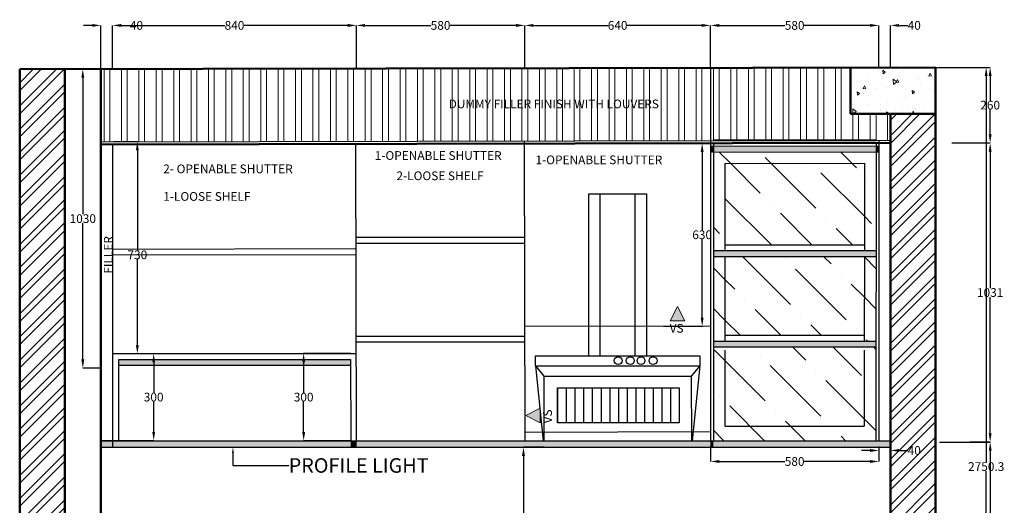
# Model space of a CAD drawing. Units: millimetres. Extents: x 26138 to 44889, y 15820 to 21179.
# Tile 4 of 8: x 31250 to 34642, y 17594 to 19266. Entities that reach past the tile are written whole.
import ezdxf
from ezdxf import colors
from ezdxf.entities.mleader import LeaderData, LeaderLine
from ezdxf.math import Vec2, Vec3

# ---------------------------------------------------------------- set-up
doc = ezdxf.new("R2010")
doc.units = ezdxf.units.MM
doc.header["$MEASUREMENT"] = 0
doc.header["$PDMODE"] = 3
for name, color, linetype, lineweight in [('A-ANNO-DIMS', 70, 'Continuous', 18), ('A-ANNO-SYMB', 1, 'Continuous', 18), ('A-ANNO-TEXT', 7, 'Continuous', 18), ('A-ELEV', 7, 'Continuous', 25), ('A-FURN-PATT', 40, 'Continuous', 13), ('A-WALL', 1, 'Continuous', 50), ('A-WALL-PATT', 8, 'Continuous', 13)]:
    doc.layers.add(name, color=color, linetype=linetype, lineweight=lineweight)
doc.styles.get("Standard").update_dxf_attribs({"font": 'arial.ttf'})
doc.dimstyles.get("Standard").update_dxf_attribs({"dimtxt": 30, "dimasz": 30, "dimexe": 0.18, "dimexo": 0.0625, "dimgap": 0.09, "dimtad": 0, "dimtih": 1, "dimtoh": 1, "dimdec": 0, "dimzin": 0, "dimdsep": 46, "dimtxsty": 'Standard', "dimcen": 0.09, "dimadec": 0, "dimazin": 0, "dimtfac": 1, "dimtdec": 0, "dimtofl": 0, "dimtmove": 0, "dimatfit": 3, "dimfxl": 1, "dimtolj": 1, "dimtzin": 0, "dimarcsym": 0})
pattern_1 = [(45, (-3504.08, -2261.207), (-39.77476, 39.77476), []), (45, (-3477.56, -2261.207), (-39.77476, 39.77476), [])]
pattern_2 = [(135, (-3504.08, -2261.21), (-192.02369, 52.3701), [246.875, -49.375, 0, -49.375])]
pattern_3 = [(90, (-379.65, -2261.21), (-60, 0), []), (90, (-359.65, -2241.21), (-60, 0), [])]

# ---------------------------------------------------------------- blocks, each defined once
blk = doc.blocks.new('*D40')
at = {"layer": 'A-ANNO-DIMS', "color": 0, "lineweight": -2, "transparency": 16777216}
for p, q in [((31499.9, 19246.8), (31469.9, 19246.8)), ((31529.9, 19096.4), (31529.9, 19247)), ((31569.9, 19096.4), (31569.9, 19247)), ((31599.9, 19246.8), (31629.9, 19246.8))]:
    blk.add_line(p, q, dxfattribs=at)
at = {"layer": 'A-ANNO-DIMS', "color": 0, "transparency": 16777216}
for points in [[(31499.9, 19251.8), (31499.9, 19241.8), (31529.9, 19246.8)], [(31599.9, 19251.8), (31599.9, 19241.8), (31569.9, 19246.8)]]:
    blk.add_solid(points, dxfattribs=at)
at = {"layer": 'Defpoints', "color": 0, "transparency": 16777216}
for p in [(31569.9, 19246.8), (31529.9, 19096.3), (31569.9, 19096.3)]:
    blk.add_point(p, dxfattribs=at)
at = {"layer": 'A-ANNO-DIMS', "color": 0, "transparency": 16777216, "insert": (31652, 19246.8), "char_height": 30, "attachment_point": 5}
blk.add_mtext('\\A1;40', dxfattribs=at)
blk = doc.blocks.new('*D41')
at = {"layer": 'A-ANNO-DIMS', "color": 0, "lineweight": -2, "transparency": 16777216}
for p, q in [((31569.9, 19096.5), (31569.9, 19247)), ((31599.9, 19246.8), (31956.7, 19246.8)), ((32379.9, 19246.8), (32023.1, 19246.8)), ((32409.9, 19096.5), (32409.9, 19247))]:
    blk.add_line(p, q, dxfattribs=at)
at = {"layer": 'A-ANNO-DIMS', "color": 0, "transparency": 16777216}
for points in [[(31599.9, 19251.8), (31599.9, 19241.8), (31569.9, 19246.8)], [(32379.9, 19251.8), (32379.9, 19241.8), (32409.9, 19246.8)]]:
    blk.add_solid(points, dxfattribs=at)
at = {"layer": 'Defpoints', "color": 0, "transparency": 16777216}
for p in [(32409.9, 19246.8), (31569.9, 19096.4), (32409.9, 19096.4)]:
    blk.add_point(p, dxfattribs=at)
at = {"layer": 'A-ANNO-DIMS', "color": 0, "transparency": 16777216, "insert": (31989.9, 19246.8), "char_height": 30, "attachment_point": 5}
blk.add_mtext('\\A1;840', dxfattribs=at)
blk = doc.blocks.new('*D42')
at = {"layer": 'A-ANNO-DIMS', "color": 0, "lineweight": -2, "transparency": 16777216}
for p, q in [((32409.9, 19098.2), (32409.9, 19247)), ((32439.9, 19246.8), (32666.7, 19246.8)), ((32959.9, 19246.8), (32733, 19246.8)), ((32989.9, 19099.5), (32989.9, 19247))]:
    blk.add_line(p, q, dxfattribs=at)
at = {"layer": 'A-ANNO-DIMS', "color": 0, "transparency": 16777216}
for points in [[(32439.9, 19251.8), (32439.9, 19241.8), (32409.9, 19246.8)], [(32959.9, 19251.8), (32959.9, 19241.8), (32989.9, 19246.8)]]:
    blk.add_solid(points, dxfattribs=at)
at = {"layer": 'Defpoints', "color": 0, "transparency": 16777216}
for p in [(32989.9, 19246.8), (32409.9, 19098.2), (32989.9, 19099.4)]:
    blk.add_point(p, dxfattribs=at)
at = {"layer": 'A-ANNO-DIMS', "color": 0, "transparency": 16777216, "insert": (32699.9, 19246.8), "char_height": 30, "attachment_point": 5}
blk.add_mtext('\\A1;580', dxfattribs=at)
blk = doc.blocks.new('*D43')
at = {"layer": 'A-ANNO-DIMS', "color": 0, "lineweight": -2, "transparency": 16777216}
for p, q in [((32989.9, 19099.5), (32989.9, 19247)), ((33019.9, 19246.8), (33276.6, 19246.8)), ((33599.9, 19246.8), (33343.1, 19246.8)), ((33629.9, 19099.5), (33629.9, 19247))]:
    blk.add_line(p, q, dxfattribs=at)
at = {"layer": 'A-ANNO-DIMS', "color": 0, "transparency": 16777216}
for points in [[(33019.9, 19251.8), (33019.9, 19241.8), (32989.9, 19246.8)], [(33599.9, 19251.8), (33599.9, 19241.8), (33629.9, 19246.8)]]:
    blk.add_solid(points, dxfattribs=at)
at = {"layer": 'Defpoints', "color": 0, "transparency": 16777216}
for p in [(33629.9, 19246.8), (32989.9, 19099.4), (33629.9, 19099.4)]:
    blk.add_point(p, dxfattribs=at)
at = {"layer": 'A-ANNO-DIMS', "color": 0, "transparency": 16777216, "insert": (33309.9, 19246.8), "char_height": 30, "attachment_point": 5}
blk.add_mtext('\\A1;640', dxfattribs=at)
blk = doc.blocks.new('*D44')
at = {"layer": 'A-ANNO-DIMS', "color": 0, "lineweight": -2, "transparency": 16777216}
for p, q in [((33629.9, 19100.8), (33629.9, 19247)), ((33659.9, 19246.8), (33886.7, 19246.8)), ((34179.9, 19246.8), (33953, 19246.8)), ((34209.9, 19102), (34209.9, 19247))]:
    blk.add_line(p, q, dxfattribs=at)
at = {"layer": 'A-ANNO-DIMS', "color": 0, "transparency": 16777216}
for points in [[(33659.9, 19251.8), (33659.9, 19241.8), (33629.9, 19246.8)], [(34179.9, 19251.8), (34179.9, 19241.8), (34209.9, 19246.8)]]:
    blk.add_solid(points, dxfattribs=at)
at = {"layer": 'Defpoints', "color": 0, "transparency": 16777216}
for p in [(34209.9, 19246.8), (33629.9, 19100.7), (34209.9, 19101.9)]:
    blk.add_point(p, dxfattribs=at)
at = {"layer": 'A-ANNO-DIMS', "color": 0, "transparency": 16777216, "insert": (33919.9, 19246.8), "char_height": 30, "attachment_point": 5}
blk.add_mtext('\\A1;580', dxfattribs=at)
blk = doc.blocks.new('*D45')
at = {"layer": 'A-ANNO-DIMS', "color": 0, "lineweight": -2, "transparency": 16777216}
for p, q in [((34179.9, 19246.8), (34149.9, 19246.8)), ((34209.9, 19102), (34209.9, 19247)), ((34249.9, 19102.1), (34249.9, 19247)), ((34279.9, 19246.8), (34309.9, 19246.8))]:
    blk.add_line(p, q, dxfattribs=at)
at = {"layer": 'A-ANNO-DIMS', "color": 0, "transparency": 16777216}
for points in [[(34179.9, 19251.8), (34179.9, 19241.8), (34209.9, 19246.8)], [(34279.9, 19251.8), (34279.9, 19241.8), (34249.9, 19246.8)]]:
    blk.add_solid(points, dxfattribs=at)
at = {"layer": 'Defpoints', "color": 0, "transparency": 16777216}
for p in [(34249.9, 19246.8), (34209.9, 19101.9), (34249.9, 19102)]:
    blk.add_point(p, dxfattribs=at)
at = {"layer": 'A-ANNO-DIMS', "color": 0, "transparency": 16777216, "insert": (34332, 19246.8), "char_height": 30, "attachment_point": 5}
blk.add_mtext('\\A1;40', dxfattribs=at)
blk = doc.blocks.new('*D46')
at = {"layer": 'A-ANNO-DIMS', "color": 0, "lineweight": -2, "transparency": 16777216}
for p, q in [((34439.1, 19102.4), (34593.8, 19102.4)), ((34593.6, 19072.4), (34593.6, 18987.6)), ((34593.6, 18872), (34593.6, 18956.8)), ((34461.3, 18842), (34593.8, 18842))]:
    blk.add_line(p, q, dxfattribs=at)
at = {"layer": 'A-ANNO-DIMS', "color": 0, "transparency": 16777216}
for points in [[(34588.6, 19072.4), (34598.6, 19072.4), (34593.6, 19102.4)], [(34588.6, 18872), (34598.6, 18872), (34593.6, 18842)]]:
    blk.add_solid(points, dxfattribs=at)
at = {"layer": 'Defpoints', "color": 0, "transparency": 16777216}
for p in [(34439, 19102.4), (34461.2, 18842), (34593.6, 18842)]:
    blk.add_point(p, dxfattribs=at)
at = {"layer": 'A-ANNO-DIMS', "color": 0, "transparency": 16777216, "insert": (34593.6, 18972.2), "char_height": 30, "attachment_point": 5}
blk.add_mtext('\\A1;260', dxfattribs=at)
blk = doc.blocks.new('*D47')
at = {"layer": 'A-ANNO-DIMS', "color": 0, "lineweight": -2, "transparency": 16777216}
for p, q in [((34461.3, 18842), (34593.8, 18842)), ((34593.6, 18812), (34593.6, 18342.2)), ((34593.6, 17841.5), (34593.6, 18311.3)), ((34419.4, 17811.5), (34593.8, 17811.5))]:
    blk.add_line(p, q, dxfattribs=at)
at = {"layer": 'A-ANNO-DIMS', "color": 0, "transparency": 16777216}
for points in [[(34588.6, 18812), (34598.6, 18812), (34593.6, 18842)], [(34588.6, 17841.5), (34598.6, 17841.5), (34593.6, 17811.5)]]:
    blk.add_solid(points, dxfattribs=at)
at = {"layer": 'Defpoints', "color": 0, "transparency": 16777216}
for p in [(34461.2, 18842), (34419.3, 17811.5), (34593.6, 17811.5)]:
    blk.add_point(p, dxfattribs=at)
at = {"layer": 'A-ANNO-DIMS', "color": 0, "transparency": 16777216, "insert": (34593.6, 18326.7), "char_height": 30, "attachment_point": 5}
blk.add_mtext('\\A1;1031', dxfattribs=at)
blk = doc.blocks.new('*D48')
at = {"layer": 'A-ANNO-DIMS', "color": 0, "lineweight": -2, "transparency": 16777216}
for p, q in [((34523.2, 17812), (34594, 17812)), ((34593.8, 17782), (34593.8, 17527.4)), ((34593.8, 17242), (34593.8, 17496.6)), ((34422.5, 17212), (34594, 17212))]:
    blk.add_line(p, q, dxfattribs=at)
at = {"layer": 'A-ANNO-DIMS', "color": 0, "transparency": 16777216}
for points in [[(34588.8, 17782), (34598.8, 17782), (34593.8, 17812)], [(34588.8, 17242), (34598.8, 17242), (34593.8, 17212)]]:
    blk.add_solid(points, dxfattribs=at)
at = {"layer": 'Defpoints', "color": 0, "transparency": 16777216}
for p in [(34523.1, 17812), (34422.5, 17212), (34593.8, 17212)]:
    blk.add_point(p, dxfattribs=at)
at = {"layer": 'A-ANNO-DIMS', "color": 0, "transparency": 16777216, "insert": (34593.8, 17512), "char_height": 30, "attachment_point": 5}
blk.add_mtext('\\A1;600', dxfattribs=at)
blk = doc.blocks.new('*D52')
at = {"layer": 'A-ANNO-DIMS', "color": 0, "lineweight": -2, "transparency": 16777216}
for p, q in [((31573.6, 18846.4), (31655.4, 18846.4)), ((31655.2, 18816.4), (31655.2, 18472)), ((31655.2, 18146.4), (31655.2, 18441.2)), ((31573.6, 18116.4), (31655.4, 18116.4))]:
    blk.add_line(p, q, dxfattribs=at)
at = {"layer": 'A-ANNO-DIMS', "color": 0, "transparency": 16777216}
for points in [[(31650.2, 18816.4), (31660.2, 18816.4), (31655.2, 18846.4)], [(31650.2, 18146.4), (31660.2, 18146.4), (31655.2, 18116.4)]]:
    blk.add_solid(points, dxfattribs=at)
at = {"layer": 'Defpoints', "color": 0, "transparency": 16777216}
for p in [(31573.5, 18846.4), (31573.5, 18116.4), (31655.2, 18116.4)]:
    blk.add_point(p, dxfattribs=at)
at = {"layer": 'A-ANNO-DIMS', "color": 0, "transparency": 16777216, "insert": (31655.2, 18456.6), "char_height": 30, "attachment_point": 5}
blk.add_mtext('\\A1;730', dxfattribs=at)
blk = doc.blocks.new('*D53')
at = {"layer": 'A-ANNO-DIMS', "color": 0, "lineweight": -2, "transparency": 16777216}
for p, q in [((33467.8, 18840.7), (33601.5, 18840.7)), ((33601.3, 18810.7), (33601.3, 18541.1)), ((33601.3, 18240.7), (33601.3, 18510.3)), ((33467.8, 18210.7), (33601.5, 18210.7))]:
    blk.add_line(p, q, dxfattribs=at)
at = {"layer": 'A-ANNO-DIMS', "color": 0, "transparency": 16777216}
for points in [[(33596.3, 18810.7), (33606.3, 18810.7), (33601.3, 18840.7)], [(33596.3, 18240.7), (33606.3, 18240.7), (33601.3, 18210.7)]]:
    blk.add_solid(points, dxfattribs=at)
at = {"layer": 'Defpoints', "color": 0, "transparency": 16777216}
for p in [(33467.7, 18840.7), (33467.7, 18210.7), (33601.3, 18210.7)]:
    blk.add_point(p, dxfattribs=at)
at = {"layer": 'A-ANNO-DIMS', "color": 0, "transparency": 16777216, "insert": (33601.3, 18525.7), "char_height": 30, "attachment_point": 5}
blk.add_mtext('\\A1;630', dxfattribs=at)
blk = doc.blocks.new('*D54')
at = {"layer": 'A-ANNO-DIMS', "color": 0, "lineweight": -2, "transparency": 16777216}
for p, q in [((33629.9, 17796.4), (33629.9, 17744.6)), ((34209.9, 17796.4), (34209.9, 17744.6)), ((33659.9, 17744.8), (33886.7, 17744.8)), ((34179.9, 17744.8), (33953, 17744.8))]:
    blk.add_line(p, q, dxfattribs=at)
at = {"layer": 'A-ANNO-DIMS', "color": 0, "transparency": 16777216}
for points in [[(33659.9, 17749.8), (33659.9, 17739.8), (33629.9, 17744.8)], [(34179.9, 17749.8), (34179.9, 17739.8), (34209.9, 17744.8)]]:
    blk.add_solid(points, dxfattribs=at)
at = {"layer": 'Defpoints', "color": 0, "transparency": 16777216}
for p in [(33629.9, 17796.4), (34209.9, 17796.4), (34209.9, 17744.8)]:
    blk.add_point(p, dxfattribs=at)
at = {"layer": 'A-ANNO-DIMS', "color": 0, "transparency": 16777216, "insert": (33919.9, 17744.8), "char_height": 30, "attachment_point": 5}
blk.add_mtext('\\A1;580', dxfattribs=at)
blk = doc.blocks.new('*D55')
at = {"layer": 'A-ANNO-DIMS', "color": 0, "lineweight": -2, "transparency": 16777216}
for p, q in [((34179.9, 17782.7), (34149.9, 17782.7)), ((34209.9, 17796.4), (34209.9, 17782.5)), ((34249.9, 17796.4), (34249.9, 17782.5)), ((34279.9, 17782.7), (34309.9, 17782.7))]:
    blk.add_line(p, q, dxfattribs=at)
at = {"layer": 'A-ANNO-DIMS', "color": 0, "transparency": 16777216}
for points in [[(34179.9, 17787.7), (34179.9, 17777.7), (34209.9, 17782.7)], [(34279.9, 17787.7), (34279.9, 17777.7), (34249.9, 17782.7)]]:
    blk.add_solid(points, dxfattribs=at)
at = {"layer": 'Defpoints', "color": 0, "transparency": 16777216}
for p in [(34209.9, 17796.4), (34249.9, 17796.4), (34249.9, 17782.7)]:
    blk.add_point(p, dxfattribs=at)
at = {"layer": 'A-ANNO-DIMS', "color": 0, "transparency": 16777216, "insert": (34332, 17782.7), "char_height": 30, "attachment_point": 5}
blk.add_mtext('\\A1;40', dxfattribs=at)
blk = doc.blocks.new('*D64')
at = {"layer": 'A-ANNO-DIMS', "color": 0, "lineweight": -2, "transparency": 16777216}
for p, q in [((33055.7, 17793.8), (32985.4, 17793.8)), ((32985.6, 17763.8), (32985.6, 17518.3)), ((32985.6, 17242), (32985.6, 17487.5)), ((33020.5, 17212), (32985.4, 17212))]:
    blk.add_line(p, q, dxfattribs=at)
at = {"layer": 'A-ANNO-DIMS', "color": 0, "transparency": 16777216}
for points in [[(32980.6, 17763.8), (32990.6, 17763.8), (32985.6, 17793.8)], [(32980.6, 17242), (32990.6, 17242), (32985.6, 17212)]]:
    blk.add_solid(points, dxfattribs=at)
at = {"layer": 'Defpoints', "color": 0, "transparency": 16777216}
for p in [(33055.8, 17793.8), (32985.6, 17212), (33020.5, 17212)]:
    blk.add_point(p, dxfattribs=at)
at = {"layer": 'A-ANNO-DIMS', "color": 0, "transparency": 16777216, "insert": (32985.6, 17502.9), "char_height": 30, "attachment_point": 5}
blk.add_mtext('\\A1;582', dxfattribs=at)
blk = doc.blocks.new('*D69')
at = {"layer": 'A-ANNO-DIMS', "color": 0, "lineweight": -2, "transparency": 16777216}
for p, q in [((32390.4, 18116.4), (32228, 18116.4)), ((32228.2, 18086.4), (32228.2, 17981.9)), ((32228.2, 17846.5), (32228.2, 17951)), ((32390.4, 17816.5), (32228, 17816.5))]:
    blk.add_line(p, q, dxfattribs=at)
at = {"layer": 'A-ANNO-DIMS', "color": 0, "transparency": 16777216}
for points in [[(32223.2, 18086.4), (32233.2, 18086.4), (32228.2, 18116.4)], [(32223.2, 17846.5), (32233.2, 17846.5), (32228.2, 17816.5)]]:
    blk.add_solid(points, dxfattribs=at)
at = {"layer": 'Defpoints', "color": 0, "transparency": 16777216}
for p in [(32390.5, 18116.4), (32228.2, 17816.5), (32390.5, 17816.5)]:
    blk.add_point(p, dxfattribs=at)
at = {"layer": 'A-ANNO-DIMS', "color": 0, "transparency": 16777216, "insert": (32228.2, 17966.5), "char_height": 30, "attachment_point": 5}
blk.add_mtext('\\A1;300', dxfattribs=at)
blk = doc.blocks.new('*D70')
at = {"layer": 'A-ANNO-DIMS', "color": 0, "lineweight": -2, "transparency": 16777216}
for p, q in [((31569.9, 18116.4), (31711.7, 18116.4)), ((31711.5, 18086.4), (31711.5, 17982.1)), ((31711.5, 17846.9), (31711.5, 17951.2)), ((31529.9, 17816.9), (31711.7, 17816.9))]:
    blk.add_line(p, q, dxfattribs=at)
at = {"layer": 'A-ANNO-DIMS', "color": 0, "transparency": 16777216}
for points in [[(31706.5, 18086.4), (31716.5, 18086.4), (31711.5, 18116.4)], [(31706.5, 17846.9), (31716.5, 17846.9), (31711.5, 17816.9)]]:
    blk.add_solid(points, dxfattribs=at)
at = {"layer": 'Defpoints', "color": 0, "transparency": 16777216}
for p in [(31569.9, 18116.4), (31711.5, 18116.4), (31529.9, 17816.9)]:
    blk.add_point(p, dxfattribs=at)
at = {"layer": 'A-ANNO-DIMS', "color": 0, "transparency": 16777216, "insert": (31711.5, 17966.6), "char_height": 30, "attachment_point": 5}
blk.add_mtext('\\A1;300', dxfattribs=at)
blk = doc.blocks.new('*D121')
at = {"layer": 'A-ANNO-DIMS', "color": 0, "lineweight": -2, "transparency": 16777216}
for p, q in [((31529.8, 19096.3), (31467.1, 19096.3)), ((31467.3, 19066.3), (31467.3, 18596.8)), ((31467.3, 18096.3), (31467.3, 18565.9)), ((31529.8, 18066.3), (31467.1, 18066.3))]:
    blk.add_line(p, q, dxfattribs=at)
at = {"layer": 'A-ANNO-DIMS', "color": 0, "transparency": 16777216}
for points in [[(31462.3, 19066.3), (31472.3, 19066.3), (31467.3, 19096.3)], [(31462.3, 18096.3), (31472.3, 18096.3), (31467.3, 18066.3)]]:
    blk.add_solid(points, dxfattribs=at)
at = {"layer": 'Defpoints', "color": 0, "transparency": 16777216}
for p in [(31529.9, 19096.3), (31467.3, 18066.3), (31529.9, 18066.3)]:
    blk.add_point(p, dxfattribs=at)
at = {"layer": 'A-ANNO-DIMS', "color": 0, "transparency": 16777216, "insert": (31467.3, 18581.3), "char_height": 30, "attachment_point": 5}
blk.add_mtext('\\A1;1030', dxfattribs=at)
blk = doc.blocks.new('SYMB-VS-TRIANGLE')
for p, q in [((0, 0), (25, 49.1)), ((50, 0), (25, 49.1)), ((0, 0), (50, 0))]:
    blk.add_line(p, q)
blk = doc.blocks.new('*D137')
at = {"layer": 'A-ANNO-DIMS', "color": 0, "lineweight": -2, "transparency": 16777216}
for p, q in [((34404.9, 19102.3), (34580, 19102.3)), ((34579.9, 19072.3), (34579.9, 17742.6)), ((34579.9, 16382), (34579.9, 17711.8)), ((34404.9, 16352), (34580, 16352))]:
    blk.add_line(p, q, dxfattribs=at)
at = {"layer": 'A-ANNO-DIMS', "color": 0, "transparency": 16777216}
for points in [[(34574.9, 19072.3), (34584.9, 19072.3), (34579.9, 19102.3)], [(34574.9, 16382), (34584.9, 16382), (34579.9, 16352)]]:
    blk.add_solid(points, dxfattribs=at)
at = {"layer": 'Defpoints', "color": 0, "transparency": 16777216}
for p in [(34404.9, 19102.3), (34404.9, 16352), (34579.9, 16352)]:
    blk.add_point(p, dxfattribs=at)
at = {"layer": 'A-ANNO-DIMS', "color": 0, "transparency": 16777216, "insert": (34579.9, 17727.2), "char_height": 30, "attachment_point": 5}
blk.add_mtext('\\A1;2750.3', dxfattribs=at)

msp = doc.modelspace()

# ---------------------------------------------------------------- hatches: boundary and pattern name
at = {"layer": 'A-FURN-PATT'}
h = msp.add_hatch(color=256, dxfattribs=at)
h.dxf.hatch_style = 1
h.paths.add_polyline_path([(33639.863, 18830.74), (33629.863, 18830.719), (33629.862, 18810.719), (33639.862, 18810.74)])
h = msp.add_hatch(color=256, dxfattribs=at)
h.dxf.hatch_style = 1
h.paths.add_polyline_path([(33639.863, 18830.74), (33639.862, 18810.74), (34200.359, 18811.907), (34200.369, 18831.907)])
h = msp.add_hatch(color=256, dxfattribs=at)
h.dxf.hatch_style = 1
h.paths.add_polyline_path([(34200.359, 18811.907), (34210.359, 18811.928), (34210.369, 18831.928), (34200.369, 18831.907)])
h = msp.add_hatch(dxfattribs=at)
h.set_pattern_fill('ANSI36', color=256, scale=790, angle=90)
h.set_pattern_definition(pattern_2)
h.paths.add_polyline_path([(34200.359, 18811.907), (33639.862, 18810.74), (33639.861, 18470.03), (33679.861, 18470.03), (33679.862, 18770.823), (34160.339, 18771.824), (34160.196, 18490.029), (34160.186, 18470.029), (34200.186, 18470.028)])
h = msp.add_hatch(dxfattribs=at)
h.set_pattern_fill('ANSI36', color=256, scale=790, angle=90)
h.set_pattern_definition(pattern_2)
h.paths.add_polyline_path([(34160.196, 18490.029), (34160.339, 18771.824), (33679.862, 18770.823), (33679.861, 18490.03)], flags=17)
h = msp.add_hatch(color=256, dxfattribs=at)
h.dxf.hatch_style = 1
h.paths.add_polyline_path([(34200.175, 18470.028), (33639.861, 18470.03), (33639.861, 18450.03), (34200.165, 18450.028)])
h = msp.add_hatch(dxfattribs=at)
h.set_pattern_fill('ANSI36', color=256, scale=790, angle=90)
h.set_pattern_definition(pattern_2)
h.paths.add_polyline_path([(33639.86, 18158.235), (33679.86, 18158.235), (33679.861, 18450.03), (33639.861, 18450.03)])
h = msp.add_hatch(dxfattribs=at)
h.set_pattern_fill('ANSI36', color=256, scale=790, angle=90)
h.set_pattern_definition(pattern_2)
h.paths.add_polyline_path([(33679.861, 18450.03), (33679.86, 18178.235), (34160.037, 18178.233), (34160.175, 18450.029)])
h = msp.add_hatch(dxfattribs=at)
h.set_pattern_fill('ANSI36', color=256, scale=790, angle=90)
h.set_pattern_definition(pattern_2)
h.paths.add_polyline_path([(34200.175, 18450.028), (34160.175, 18450.029), (34160.037, 18178.233), (34160.027, 18158.233), (34200.027, 18158.233)])
h = msp.add_hatch(color=256, dxfattribs=at)
h.dxf.hatch_style = 1
h.paths.add_polyline_path([(33491.544, 18229.434), (33541.544, 18229.434), (33516.544, 18278.526)])
h = msp.add_hatch(color=256, dxfattribs=at)
h.dxf.hatch_style = 1
h.paths.add_polyline_path([(34200.012, 18138.233), (34200.022, 18158.233), (33639.86, 18158.235), (33639.86, 18138.235)])
h = msp.add_hatch(dxfattribs=at)
h.set_pattern_fill('ANSI36', color=256, scale=790, angle=90)
h.set_pattern_definition(pattern_2)
h.paths.add_polyline_path([(34199.844, 17816.438), (34200.01, 18138.233), (33639.86, 18138.235), (33639.859, 17816.438)])
h = msp.add_hatch(color=256, dxfattribs=at)
h.dxf.hatch_style = 1
h.paths.add_polyline_path([(31589.864, 18096.438), (31589.864, 18076.438), (32389.907, 18076.438), (32389.864, 18096.438)])
h = msp.add_hatch(color=256, dxfattribs=at)
h.dxf.hatch_style = 1
h.paths.add_polyline_path([(33042.594, 17878.319), (33042.594, 17928.319), (32993.502, 17903.319)])
h = msp.add_hatch(color=256, dxfattribs=at)
h.dxf.hatch_style = 1
h.paths.add_polyline_path([(32390.468, 17816.438), (31529.862, 17816.438), (31529.862, 17793.785), (32390.517, 17793.785)])
h = msp.add_hatch(color=256, dxfattribs=at)
h.dxf.hatch_style = 1
h.paths.add_polyline_path([(32410.473, 17816.438), (32390.473, 17816.389), (32390.517, 17793.785), (32410.515, 17793.785)])
h = msp.add_hatch(color=256, dxfattribs=at)
h.dxf.hatch_style = 1
h.paths.add_polyline_path([(32989.823, 17816.438), (32410.468, 17816.438), (32410.515, 17793.785), (32989.869, 17793.785)])
h = msp.add_hatch(color=256, dxfattribs=at)
h.dxf.hatch_style = 1
h.paths.add_polyline_path([(33055.779, 17816.438), (32989.815, 17816.372), (32989.869, 17793.785), (33055.779, 17793.785), (33055.779, 17795.785)])
h = msp.add_hatch(color=256, dxfattribs=at)
h.dxf.hatch_style = 1
h.paths.add_polyline_path([(33564.442, 17796.305), (33564.401, 17816.438), (33055.779, 17816.438), (33055.779, 17795.785), (33055.779, 17793.785), (33564.185, 17793.785)])
h = msp.add_hatch(color=256, dxfattribs=at)
h.dxf.hatch_style = 1
h.paths.add_polyline_path([(33629.859, 17816.438), (33563.381, 17816.309), (33564.442, 17796.305), (33563.412, 17793.785), (33629.859, 17793.785)])
h = msp.add_hatch(color=256, dxfattribs=at)
h.dxf.hatch_style = 1
h.paths.add_polyline_path([(33639.859, 17816.438), (33629.859, 17816.438), (33629.859, 17793.785), (33639.859, 17793.785)])
h = msp.add_hatch(color=256, dxfattribs=at)
h.dxf.hatch_style = 1
h.paths.add_polyline_path([(33639.859, 17816.438), (33639.859, 17793.785), (34249.853, 17793.785), (34249.865, 17816.438)])
at = {"layer": 'A-WALL-PATT'}
h = msp.add_hatch(dxfattribs=at)
h.set_pattern_fill('ANSI32', color=256, scale=160, angle=45)
h.set_pattern_definition(pattern_3)
h.paths.add_polyline_path([(33629.863, 18850.72), (33629.864, 19100.72), (31529.865, 19096.348), (31529.864, 18846.347)])
h.paths.add_polyline_path([(32720.06, 18953.058), (33527.288, 18953.058), (33527.288, 18999.623), (32720.06, 18999.623)], flags=24)
h = msp.add_hatch(dxfattribs=at)
h.set_pattern_fill('ANSI32', color=256, scale=160, angle=45)
h.set_pattern_definition(pattern_3)
h.paths.add_polyline_path([(33629.864, 19100.72), (33629.863, 18850.72), (34249.859, 18852.01), (34249.859, 18942.01), (34112.394, 18942.01), (34112.394, 19101.725)])
h = msp.add_hatch(dxfattribs=at)
h.set_pattern_fill('AR-CONC', color=256, scale=16, angle=45)
h.set_pattern_definition([(95, (-3504.08, -2261.21), (88.24832, 74.04913), [12, -132]), (40, (-3504.08, -2261.21), (-100.79875, 69.4029), [9.6, -105.6]), (145.45144, (-3496.72, -2255.04), (-12.55043, 143.45204), [10.19843, -112.18274]), (91.1842, (-3526.7, -2238.58), (139.47094, 102.0182), [18, -198]), (141.63564, (-3515.08, -2230.08), (-4.464, 215.95387), [15.29765, -168.2742]), (36.18416, (-3526.7, -2238.58), (-4.464, 215.9539), [14.4, -158.4]), (66, (-3509.74, -2232.92), (113.08345, 21.9812), [12, -132]), (11, (-3509.74, -2232.92), (-54.51337, 109.56935), [9.6, -105.6]), (116.45144, (-3500.31, -2231.09), (58.57008, 131.55054), [10.19843, -112.18274]), (82.5, (-3504.08, -2261.207), (-36.28691, 39.03837), [0, -104.32, 0, -107.2, 0, -106]), (52.5, (-3504.08, -2261.207), (-14.85967, 74.38551), [0, -61.12, 0, -101.92, 0, -40.4]), (12.5, (-3529.31, -2286.437), (62.946907, 57.84332), [0, -40, 0, -124.8, 0, -165.6]), (2.5, (-3540.62, -2297.75), (54.6544, 77.30557), [0, -52, 0, -82.88, 0, -117.6])])
h.paths.add_polyline_path([(34404.859, 19102.011), (34249.859, 19102.011), (34112.394, 19101.725), (34112.394, 18942.01), (34404.859, 18942.01)])
h = msp.add_hatch(dxfattribs=at)
h.set_pattern_fill('ANSI32', color=256, scale=150)
h.set_pattern_definition(pattern_1)
h.paths.add_polyline_path([(31404.865, 19096.088), (31249.865, 19095.765), (31249.859, 16352.011), (31404.859, 16352.011)])
h = msp.add_hatch(dxfattribs=at)
h.set_pattern_fill('ANSI32', color=256, scale=150)
h.set_pattern_definition(pattern_1)
h.paths.add_polyline_path([(34404.859, 18942.01), (34249.859, 18942.01), (34249.859, 16352.011), (34404.859, 16352.011)])

# ---------------------------------------------------------------- linework, layer by layer
at = {"layer": 'A-ANNO-SYMB'}
for p in [(34160.186, 18490.029), (32989.154, 18157.42), (34160.032, 18178.233)]:
    msp.add_point(p, dxfattribs=at)
at = {"layer": 'A-ELEV'}
for p, q in [((33629.864, 19100.72), (33629.859, 17816.588)), ((31530.385, 18846.349), (34250.379, 18852.011)), ((31569.864, 18836.431), (31569.864, 18116.438)), ((32410.468, 17816.255), (32408.341, 18838.176)), ((32987.713, 18849.383), (32989.814, 17816.576)), ((33629.863, 18830.719), (34210.369, 18831.928)), ((33639.863, 18840.74), (33639.859, 17816.438)), ((33639.863, 18840.74), (34200.374, 18841.907)), ((34200.374, 18841.907), (34199.844, 17816.438)), ((34210.379, 18852.032), (34209.854, 17816.53)), ((33629.862, 18810.719), (34210.359, 18811.928)), ((33679.862, 18770.823), (33679.861, 18470.03)), ((33679.862, 18770.823), (34160.339, 18771.824)), ((34160.339, 18771.824), (34160.186, 18470.029)), ((33210.441, 18666.164), (33409.284, 18666.164)), ((33210.441, 18108.977), (33210.441, 18666.164)), ((33250.441, 18108.977), (33250.441, 18666.164)), ((33369.284, 18666.164), (33369.284, 18108.977)), ((33409.284, 18666.164), (33409.284, 18108.977)), ((32409.051, 18517.195), (32988.405, 18517.195)), ((32409.051, 18497.195), (32988.446, 18497.195)), ((34160.186, 18490.029), (33679.861, 18490.03)), ((34160.186, 18490.029), (34160.185, 18470.029)), ((31569.864, 18476.435), (32409.09, 18478.182)), ((31569.906, 18456.435), (32409.132, 18458.182)), ((34200.175, 18470.028), (33639.861, 18470.03)), ((34200.165, 18450.028), (33639.861, 18450.03)), ((33679.861, 18450.03), (33679.86, 18158.235)), ((34160.175, 18450.029), (34160.027, 18158.233)), ((33629.86, 18210.719), (32989.02, 18209.742)), ((32409.051, 18176.712), (32989.113, 18176.712)), ((32409.051, 18156.712), (32989.155, 18156.712)), ((34200.022, 18158.233), (33639.86, 18158.235)), ((34160.032, 18178.233), (33679.86, 18178.235)), ((31569.864, 18116.438), (32409.864, 18116.438)), ((31569.864, 18116.438), (31569.864, 17793.785)), ((34200.012, 18138.233), (33639.86, 18138.235)), ((33679.86, 18128.235), (33679.859, 17866.438)), ((34160.012, 18128.233), (34159.879, 17866.438)), ((31589.864, 18096.438), (32389.864, 18096.438)), ((31589.864, 18096.438), (31589.864, 17816.943)), ((32389.864, 18096.438), (32390.468, 17816.486)), ((31589.864, 18076.438), (32389.864, 18076.438)), ((33026.989, 18073.977), (33592.736, 18073.977)), ((33026.989, 18073.977), (33055.779, 18038.977)), ((33026.989, 18073.977), (33053.641, 17816.438)), ((33592.736, 18073.977), (33563.946, 18038.977)), ((33592.736, 18073.977), (33566.493, 17816.438)), ((33055.779, 18038.977), (33563.946, 18038.977)), ((33055.779, 18038.977), (33055.779, 17816.438)), ((33563.946, 18038.977), (33564.401, 17816.438)), ((33103.009, 17998.375), (33103.009, 17877.9)), ((33132.971, 17998.375), (33132.971, 17877.9)), ((33162.933, 17998.375), (33162.933, 17877.9)), ((33192.895, 17998.375), (33192.895, 17877.9)), ((33222.857, 17998.375), (33222.857, 17877.9)), ((33252.819, 17998.375), (33252.819, 17877.9)), ((33282.781, 17998.375), (33282.781, 17877.9)), ((33312.743, 17998.375), (33312.743, 17877.9)), ((33342.706, 17998.375), (33342.706, 17877.9)), ((33372.668, 17998.375), (33372.668, 17877.9)), ((33402.63, 17998.375), (33402.63, 17877.9)), ((33432.592, 17998.375), (33432.592, 17877.9)), ((33462.554, 17998.375), (33462.554, 17877.9)), ((33492.516, 17998.375), (33492.516, 17877.9)), ((33629.757, 17846.438), (32989.764, 17845.131)), ((33679.859, 17866.438), (34159.879, 17866.438)), ((31529.983, 17816.438), (34249.859, 17816.438)), ((32989.782, 17836.438), (32989.864, 17836.438)), ((33639.859, 17816.438), (34199.859, 17816.438)), ((31529.862, 17793.781), (34249.859, 17793.785)), ((33629.859, 17793.785), (34249.859, 17793.785))]:
    msp.add_line(p, q, dxfattribs=at)
msp.add_lwpolyline([(33026.989, 18073.977), (33026.989, 18108.977), (33592.736, 18108.977), (33592.736, 18073.977)], dxfattribs=at)
msp.add_lwpolyline([(33103.009, 17998.375), (33522.478, 17998.375), (33522.478, 17877.9), (33103.009, 17877.9)], close=True, dxfattribs=at)
for centre in [(33311.9, 18092.185), (33353.453, 18092.185), (33390.573, 18092.185), (33432.18, 18092.185)]:
    msp.add_circle(centre, 13.516, dxfattribs=at)
at = {"layer": 'A-WALL'}
for p, q in [((31249.865, 19095.765), (34404.859, 19102.334)), ((34112.394, 19101.725), (34112.394, 18942.01)), ((34404.859, 19102.334), (34404.859, 16352.011)), ((31249.859, 16352.011), (31249.865, 19096.349)), ((31404.859, 16352.011), (31404.865, 19096.348)), ((31529.859, 16352.011), (31529.865, 19096.348)), ((34112.394, 18942.01), (34404.859, 18942.01)), ((34249.859, 18942.01), (34249.859, 16352.011)), ((31530.406, 18836.349), (34250.4, 18842.011)), ((33639.842, 18850.74), (34200.353, 18851.907)), ((34250.379, 18852.011), (34249.859, 17826.438))]:
    msp.add_line(p, q, dxfattribs=at)

# ---------------------------------------------------------------- block references
at = {"layer": 'A-ANNO-SYMB'}
msp.add_blockref('SYMB-VS-TRIANGLE', (33491.544, 18229.434), dxfattribs=at)
at = {"layer": 'A-ANNO-SYMB', "rotation": 90.00000000001273}
msp.add_blockref('SYMB-VS-TRIANGLE', (33042.594, 17878.319), dxfattribs=at)

# ---------------------------------------------------------------- texts
at = {"layer": 'A-ANNO-TEXT'}
for s, p in [('DUMMY FILLER FINISH WITH LOUVERS', (32727.821, 18961.33)), ('1-OPENABLE SHUTTER', (32473.121, 18783.665)), ('1-OPENABLE SHUTTER', (33027.05, 18768.684)), ('2- OPENABLE SHUTTER', (31744.465, 18737.741)), ('2-LOOSE SHELF', (32547.946, 18713.816)), ('1-LOOSE SHELF', (31744.465, 18642.707)), ('VS', (33489.306, 18188.395))]:
    msp.add_text(s, height=30, dxfattribs=at).set_placement(p)
for s, p in [('FILLER', (31569.864, 18391.823)), ('VS', (33083.633, 17876.081))]:
    msp.add_text(s, height=30, rotation=90, dxfattribs=at).set_placement(p)

# ---------------------------------------------------------------- dimensions: what is measured, and where the dimension line sits
at = {"layer": 'A-ANNO-DIMS'}
for base, p1, p2, picture, middle in [((31569.865, 19246.795), (31529.865, 19096.348), (31569.865, 19096.348), '*D40', (31651.994, 19246.795)), ((32409.865, 19246.795), (31569.865, 19096.431), (32409.865, 19096.431), '*D41', (31989.865, 19246.795)), ((32989.864, 19246.795), (32409.865, 19098.18), (32989.864, 19099.388), '*D42', (32699.864, 19246.795)), ((33629.864, 19246.795), (32989.864, 19099.388), (33629.864, 19099.388), '*D43', (33309.864, 19246.795)), ((34209.861, 19246.795), (33629.864, 19100.72), (34209.861, 19101.928), '*D44', (33919.862, 19246.795)), ((34249.859, 19246.795), (34209.861, 19101.928), (34249.859, 19102.011), '*D45', (34331.988, 19246.795)), ((34249.859, 17782.665), (34209.859, 17796.438), (34249.859, 17796.438), '*D55', (34331.988, 17782.665))]:
    dim = msp.add_linear_dim(base=base, p1=p1, p2=p2, dimstyle='Standard', override={"dimclrd": 0, "dimclre": 0, "dimclrt": 0}, dxfattribs=at)
    dim.commit()
    dim.dimension.update_dxf_attribs({"geometry": picture, "text_midpoint": middle})
for base, p1, p2, override, picture, middle in [((34579.859, 16352.011), (34404.859, 19102.334), (34404.859, 16352.011), {"dimdec": 1, "dimlfac": 1, "dimrnd": 0, "dimzin": 0, "dimdsep": 46, "dimlunit": 2}, '*D137', (34579.859, 17727.172)), ((34593.609, 18842.011), (34439.022, 19102.405), (34461.188, 18842.011), {"dimclrd": 0, "dimclre": 0, "dimclrt": 0}, '*D46', (34593.609, 18972.208)), ((31467.291, 18066.348), (31529.865, 19096.348), (31529.865, 18066.348), {"dimclrd": 0, "dimclre": 0, "dimclrt": 0}, '*D121', (31467.291, 18581.348)), ((33601.325, 18210.719), (33467.705, 18840.719), (33467.705, 18210.719), {"dimclrd": 0, "dimclre": 0, "dimclrt": 0}, '*D53', (33601.325, 18525.719)), ((34593.609, 17811.46), (34461.188, 18842.011), (34419.336, 17811.46), {"dimclrd": 0, "dimclre": 0, "dimclrt": 0}, '*D47', (34593.609, 18326.735)), ((31711.501, 18116.438), (31529.862, 17816.854), (31569.864, 18116.438), {"dimclrd": 0, "dimclre": 0, "dimclrt": 0}, '*D70', (31711.501, 17966.646)), ((32228.159, 17816.486), (32390.468, 18116.438), (32390.468, 17816.486), {"dimclrd": 0, "dimclre": 0, "dimclrt": 0}, '*D69', (32228.159, 17966.462)), ((34593.789, 17212.011), (34523.108, 17812.011), (34422.485, 17212.011), {"dimclrd": 0, "dimclre": 0, "dimclrt": 0}, '*D48', (34593.789, 17512.011))]:
    dim = msp.add_linear_dim(base=base, p1=p1, p2=p2, angle=90, dimstyle='Standard', override=override, dxfattribs=at)
    dim.commit()
    dim.dimension.update_dxf_attribs({"geometry": picture, "text_midpoint": middle})
for base, p1, p2, picture, middle in [((31655.212, 18116.438), (31573.53, 18846.438), (31573.53, 18116.438), '*D52', (31655.212, 18456.612)), ((32985.563, 17212.011), (33055.779, 17793.785), (33020.55, 17212.011), '*D64', (32985.563, 17502.898))]:
    dim = msp.add_linear_dim(base=base, p1=p1, p2=p2, angle=90, dimstyle='Standard', override={"dimclrd": 0, "dimclre": 0, "dimclrt": 0}, dxfattribs=at)
    dim.commit()
    dim.dimension.update_dxf_attribs({"geometry": picture, "text_midpoint": middle, "dimtype": 160})
dim = msp.add_linear_dim(base=(34209.859, 17744.758), p1=(33629.859, 17796.438), p2=(34209.859, 17796.438), dimstyle='Standard', override={"dimclrd": 0, "dimclre": 0, "dimclrt": 0}, dxfattribs=at)
dim.commit()
dim.dimension.update_dxf_attribs({"geometry": '*D54', "text_midpoint": (33919.859, 17744.758), "dimtype": 160})

# ---------------------------------------------------------------- leaders
at = {"layer": 'A-ANNO-TEXT'}
ml = msp.add_multileader_mtext('Standard', dxfattribs=at)
ml.set_content('PROFILE LIGHT ', color=256)
ml.set_leader_properties()
ml.build(insert=Vec2(0, 0))
ml.multileader.update_dxf_attribs({"dogleg_length": 0.36, "arrow_head_size": 20})
ctx = ml.context
ctx.base_point, ctx.char_height, ctx.arrow_head_size, ctx.landing_gap_size, ctx.plane_origin = Vec3(32176.619, 17730.654), 50, 20, 0.09, Vec3(32176.259, 17730.654)
notes = []
notes.append((ctx, [(0, (1, 1, 0), (32176.259, 17730.654), (1, 0), 0.36, [(0, [(31984.581, 17793.782), (31984.581, 17730.654)], 0, [])])]))
ctx.mtext.insert, ctx.mtext.flow_direction = Vec3(32176.709, 17756.08), 5
for ctx, leaders in notes:
    for number, flags, end, landing, length, lines in leaders:
        leader = LeaderData()
        leader.index, (leader.has_last_leader_line, leader.has_dogleg_vector, leader.attachment_direction) = number, flags
        leader.last_leader_point, leader.dogleg_vector, leader.dogleg_length = Vec3(end), Vec3(landing), length
        for number, points, colour, breaks in lines:
            line = LeaderLine()
            line.index, line.vertices, line.color, line.breaks = number, Vec3.list(points), colors.encode_raw_color(colour), breaks
            leader.lines.append(line)
        ctx.leaders.append(leader)

doc.saveas('drawing.dxf')
